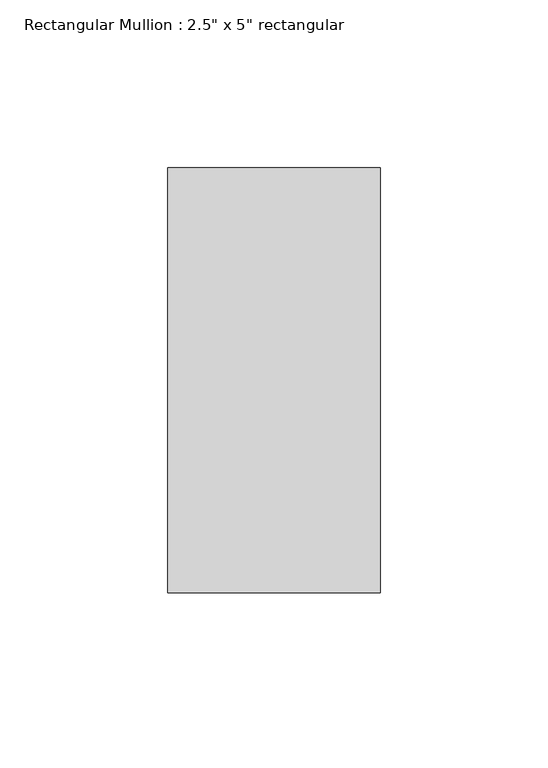
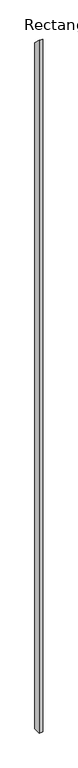
"""IFC4 building model written with IfcOpenShell, lengths in millimetres: member geometry."""

from ifc_helpers import new_model, si_unit, frame, origin, place, context, project, spatial, polyline, outline, extrude, source, transform, mapped, element, save


def member_e6b7cb81(model_context):
    return source(origin(), model_context, "Body", "SweptSolid", [
        extrude(outline(polyline([(-63.5, 63.5), (63.5, -63.5), (63.5, -12740.4663275), (-63.5, -12740.4663275), (-63.5, 63.5)])), frame((-63.5, 0.0, 0.0), z_axis=(1.0, 0.0, 0.0), x_axis=(0.0, 1.0, 0.0)), (0.0, 0.0, 1.0), 63.5),
    ])


if __name__ == "__main__":
    model = new_model("IFC4")
    model_context = context("Model", 3, world=origin())
    ifc_project = project(units=[si_unit("LENGTHUNIT", "METRE", prefix="MILLI")], contexts=[model_context])
    site = spatial("IfcSite", under=ifc_project)
    building = spatial("IfcBuilding", under=site)
    placement = place(None, origin())
    member_shape = member_e6b7cb81(model_context)
    element("IfcMember", 1, ObjectType="Rectangular Mullion : 2.5\" x 5\" rectangular", at=placement, inside=building, context=model_context, shape_type="MappedRepresentation", body=[
        mapped(member_shape, transform((0.0, 0.0, 0.0), x_axis=(1.0, 0.0, 0.0), y_axis=(0.0, 1.0, 0.0), z_axis=(0.0, 0.0, 1.0))),
    ])
    save(model, "model.ifc")

# Revit data of these elements
# Type "Rectangular Mullion : 2.5\" x 5\" rectangular"
#   built-in parameter 1007304 = 0.416667 (stored number, unit not read)
#   built-in parameter 1007301 = 0.104167 (stored number, unit not read)
#   built-in parameter 1007300 = 0.104167 (stored number, unit not read)
# Element 1 (IfcMember, "Rectangular Mullion : 2.5\" x 5\" rectangular")
#   Materials on its faces: "Aluminum"
# Materials
#   "Aluminum": class "Metal", colour RGB 247 247 247, transparency 0, Description = "Aluminum 6061", Cost = 0
